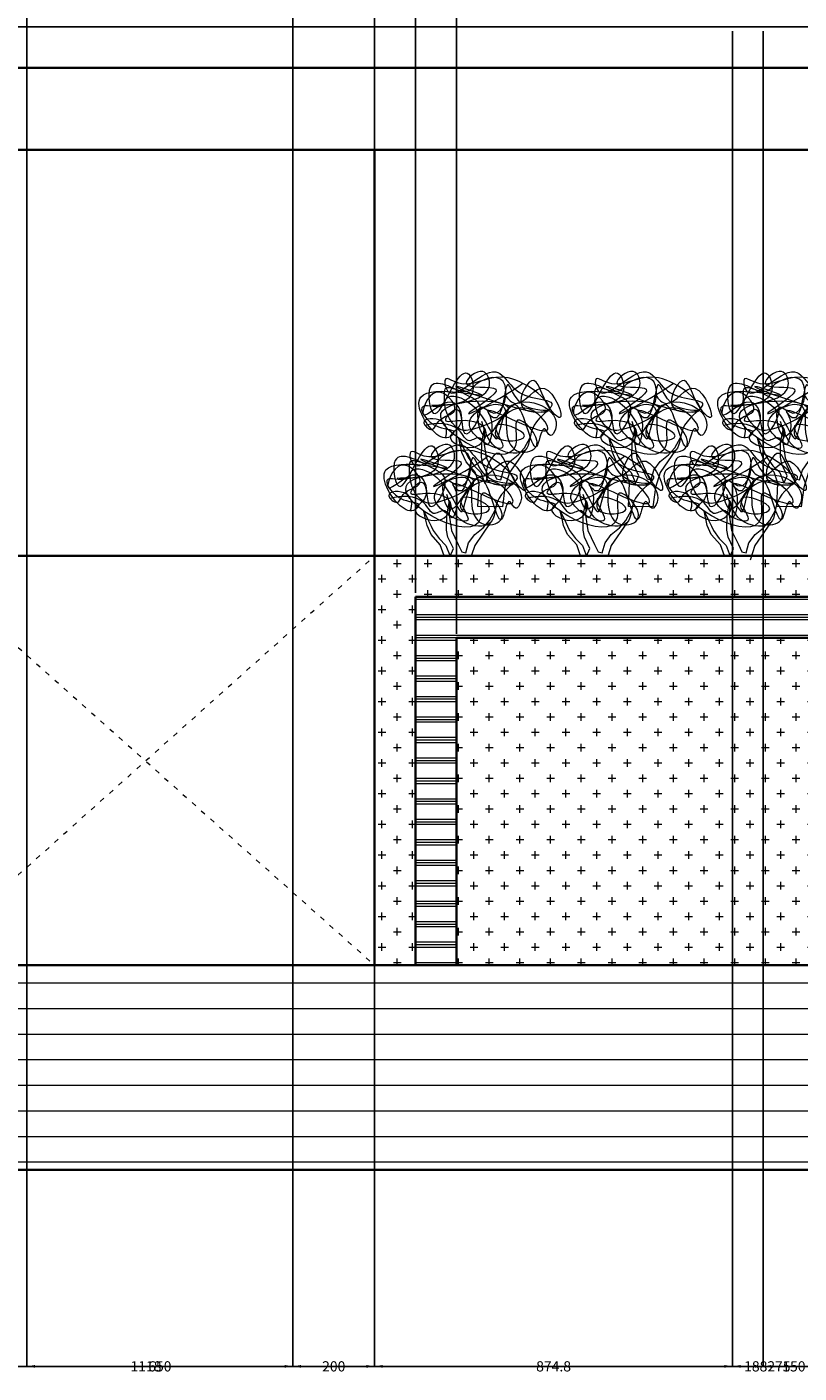
# Model space of a CAD drawing. Units: millimetres. Extents: x -692 to 9639, y -141 to 10345.
# Tile 6 of 19: x 6042 to 7929, y -141 to 3148. Entities that reach past the tile are written whole.
import ezdxf

# ---------------------------------------------------------------- set-up
doc = ezdxf.new("R2010")
doc.units = ezdxf.units.MM
doc.header["$MEASUREMENT"] = 0
doc.linetypes.add('ACAD_ISO03W100', pattern=[30, 12, -18])
for name, color, linetype, lineweight in [('A-ANNO-DIMS', 2, 'Continuous', 18), ('A-DOOR-SWNG', 3, 'ACAD_ISO03W100', 18), ('A-ELEV', 7, 'Continuous', 35), ('A-ELEV-PATT', 8, 'Continuous', 13), ('L-PLNT', 3, 'Continuous', 18)]:
    doc.layers.add(name, color=color, linetype=linetype, lineweight=lineweight)
doc.styles.get("Standard").update_dxf_attribs({"font": 'arial.ttf'})
doc.dimstyles.get("Standard").update_dxf_attribs({"dimtxt": 25, "dimasz": 20, "dimexe": 0.18, "dimexo": 10, "dimgap": 10, "dimtad": 0, "dimtih": 1, "dimtoh": 1, "dimdec": 0, "dimzin": 0, "dimdsep": 46, "dimtxsty": 'Standard', "dimcen": 10, "dimadec": 0, "dimazin": 0, "dimtfac": 1, "dimtdec": 0, "dimtofl": 0, "dimtmove": 0, "dimatfit": 3, "dimfxl": 1, "dimtolj": 1, "dimtzin": 0, "dimarcsym": 0})

# ---------------------------------------------------------------- blocks, each defined once
blk = doc.blocks.new('SHRUB-A')
for p, q in [((4.3, 148.6), (0, 167.6)), ((0, 167.6), (10, 146.8)), ((56.2, 156.7), (63.1, 192.4)), ((63.1, 192.4), (61.6, 157.6)), ((160.6, 144.2), (174.3, 169.5)), ((7.9, 132.5), (4.3, 148.6)), ((17.8, 109.9), (7.9, 132.5)), ((10, 146.8), (18, 130.3)), ((55.6, 120.9), (56.2, 156.7)), ((61.6, 157.6), (67.3, 119.6)), ((162.4, 138.4), (124.4, 83.7)), ((145.1, 126.5), (160.6, 144.2)), ((40.2, 84.8), (17.8, 109.9)), ((18, 130.3), (22.9, 120.3)), ((22.9, 120.3), (37.4, 100.1)), ((37.4, 100.1), (54, 83.6)), ((59.1, 104.1), (55.6, 120.9)), ((72.4, 75.8), (59.1, 104.1)), ((67.3, 119.6), (83.9, 86)), ((109.4, 89.7), (124.8, 110.5)), ((124.8, 110.5), (145.1, 126.5)), ((49.7, 57.7), (40.2, 84.8)), ((54, 83.6), (64.1, 57.4)), ((64.1, 57.4), (72.4, 75.8)), ((83.9, 86), (92.7, 68.2)), ((92.7, 68.2), (102.6, 65.4)), ((102.6, 65.4), (109.4, 89.7)), ((124.4, 83.7), (113, 47.4)), ((47, 0.4), (49.7, 57.7)), ((113, 47.4), (106.7, 0)), ((106.7, 0), (47, 0.4))]:
    blk.add_line(p, q)
blk = doc.blocks.new('SHRUB-B')
for p, q in [((56.2, 99.2), (63.1, 135)), ((63.1, 135), (61.6, 100.2)), ((4.3, 91.2), (0, 110.2)), ((0, 110.2), (10, 89.4)), ((55.6, 63.5), (56.2, 99.2)), ((61.6, 100.2), (67.3, 62.2)), ((160.6, 86.8), (174.3, 112.1)), ((7.9, 75.1), (4.3, 91.2)), ((17.8, 52.5), (7.9, 75.1)), ((10, 89.4), (18, 72.9)), ((18, 72.9), (22.9, 62.9)), ((124.8, 53.1), (145.1, 69.1)), ((145.1, 69.1), (160.6, 86.8)), ((40.2, 27.4), (17.8, 52.5)), ((22.9, 62.9), (37.4, 42.7)), ((37.4, 42.7), (54, 26.2)), ((59.1, 46.7), (55.6, 63.5)), ((72.4, 18.4), (59.1, 46.7)), ((67.3, 62.2), (83.9, 28.6)), ((109.4, 32.3), (124.8, 53.1)), ((49.7, 0.3), (40.2, 27.4)), ((54, 26.2), (64.1, 0)), ((64.1, 0), (72.4, 18.4)), ((83.9, 28.6), (92.7, 10.8)), ((92.7, 10.8), (102.6, 8)), ((102.6, 8), (109.4, 32.3))]:
    blk.add_line(p, q)
blk = doc.blocks.new('*D6')
at = {"layer": 'A-ANNO-DIMS', "color": 0, "lineweight": -2, "transparency": 16777216}
for p, q in [((2473.7, 345.6), (2473.7, -124.6)), ((9073.7, 345.6), (9073.7, -124.6)), ((2493.7, -124.4), (5726.4, -124.4)), ((9053.7, -124.4), (5821.1, -124.4))]:
    blk.add_line(p, q, dxfattribs=at)
at = {"layer": 'A-ANNO-DIMS', "color": 0, "lineweight": -3, "transparency": 16777216}
for points in [[(2493.7, -121.1), (2493.7, -127.8), (2473.7, -124.4)], [(9053.7, -121.1), (9053.7, -127.8), (9073.7, -124.4)]]:
    blk.add_solid(points, dxfattribs=at)
at = {"layer": 'Defpoints', "color": 0, "lineweight": -3, "transparency": 16777216}
for p in [(2473.7, 355.6), (9073.7, 355.6), (9073.7, -124.4)]:
    blk.add_point(p, dxfattribs=at)
at = {"layer": 'A-ANNO-DIMS', "color": 0, "transparency": 16777216, "insert": (5773.7, -124.4), "char_height": 25, "attachment_point": 5}
blk.add_mtext('\\A1;6600', dxfattribs=at)
blk = doc.blocks.new('*D7')
at = {"layer": 'A-ANNO-DIMS', "color": 0, "lineweight": -2, "transparency": 16777216}
for p, q in [((8481.5, 9848.8), (-649.1, 9848.8)), ((-648.9, 9828.8), (-648.9, 5124.9)), ((-648.9, 375.6), (-648.9, 5079.4)), ((2463.7, 355.6), (-649.1, 355.6))]:
    blk.add_line(p, q, dxfattribs=at)
at = {"layer": 'A-ANNO-DIMS', "color": 0, "lineweight": -3, "transparency": 16777216}
for points in [[(-652.2, 9828.8), (-645.6, 9828.8), (-648.9, 9848.8)], [(-652.2, 375.6), (-645.6, 375.6), (-648.9, 355.6)]]:
    blk.add_solid(points, dxfattribs=at)
at = {"layer": 'Defpoints', "color": 0, "lineweight": -3, "transparency": 16777216}
for p in [(-648.9, 9848.8), (8491.5, 9848.8), (2473.7, 355.6)]:
    blk.add_point(p, dxfattribs=at)
at = {"layer": 'A-ANNO-DIMS', "color": 0, "transparency": 16777216, "insert": (-648.9, 5102.2), "char_height": 25, "attachment_point": 5}
blk.add_mtext('\\A1;9493', dxfattribs=at)
blk = doc.blocks.new('*D22')
at = {"layer": 'A-ANNO-DIMS', "color": 0, "lineweight": -2, "transparency": 16777216}
for p, q in [((5773.7, 845.6), (5773.7, -124.6)), ((6891.7, 845.6), (6891.7, -124.6)), ((5793.7, -124.4), (6286.6, -124.4)), ((6871.7, -124.4), (6378.9, -124.4))]:
    blk.add_line(p, q, dxfattribs=at)
at = {"layer": 'A-ANNO-DIMS', "color": 0, "lineweight": -3, "transparency": 16777216}
for points in [[(5793.7, -121.1), (5793.7, -127.8), (5773.7, -124.4)], [(6871.7, -121.1), (6871.7, -127.8), (6891.7, -124.4)]]:
    blk.add_solid(points, dxfattribs=at)
at = {"layer": 'Defpoints', "color": 0, "lineweight": -3, "transparency": 16777216}
for p in [(5773.7, 855.6), (6891.7, 855.6), (6891.7, -124.4)]:
    blk.add_point(p, dxfattribs=at)
at = {"layer": 'A-ANNO-DIMS', "color": 0, "transparency": 16777216, "insert": (6332.7, -124.4), "char_height": 25, "attachment_point": 5}
blk.add_mtext('\\A1;1118', dxfattribs=at)
blk = doc.blocks.new('*D23')
at = {"layer": 'A-ANNO-DIMS', "color": 0, "lineweight": -2, "transparency": 16777216}
for p, q in [((6891.7, 845.6), (6891.7, -124.6)), ((8773.7, 845.6), (8773.7, -124.6)), ((6911.7, -124.4), (7786.7, -124.4)), ((8753.7, -124.4), (7878.8, -124.4))]:
    blk.add_line(p, q, dxfattribs=at)
at = {"layer": 'A-ANNO-DIMS', "color": 0, "lineweight": -3, "transparency": 16777216}
for points in [[(6911.7, -121.1), (6911.7, -127.8), (6891.7, -124.4)], [(8753.7, -121.1), (8753.7, -127.8), (8773.7, -124.4)]]:
    blk.add_solid(points, dxfattribs=at)
at = {"layer": 'Defpoints', "color": 0, "lineweight": -3, "transparency": 16777216}
for p in [(6891.7, 855.6), (8773.7, 855.6), (8773.7, -124.4)]:
    blk.add_point(p, dxfattribs=at)
at = {"layer": 'A-ANNO-DIMS', "color": 0, "transparency": 16777216, "insert": (7832.7, -124.4), "char_height": 25, "attachment_point": 5}
blk.add_mtext('\\A1;1882', dxfattribs=at)
blk = doc.blocks.new('*D32')
at = {"layer": 'A-ANNO-DIMS', "color": 0, "lineweight": -2, "transparency": 16777216}
for p, q in [((6871.7, 10328.8), (6851.7, 10328.8)), ((6891.7, 1865.6), (6891.7, 10329)), ((6991.7, 1765.6), (6991.7, 10329)), ((7011.7, 10328.8), (7031.7, 10328.8))]:
    blk.add_line(p, q, dxfattribs=at)
at = {"layer": 'A-ANNO-DIMS', "color": 0, "lineweight": -3, "transparency": 16777216}
for points in [[(6871.7, 10332.1), (6871.7, 10325.4), (6891.7, 10328.8)], [(7011.7, 10332.1), (7011.7, 10325.4), (6991.7, 10328.8)]]:
    blk.add_solid(points, dxfattribs=at)
at = {"layer": 'Defpoints', "color": 0, "lineweight": -3, "transparency": 16777216}
for p in [(6991.7, 10328.8), (6891.7, 1855.6), (6991.7, 1755.6)]:
    blk.add_point(p, dxfattribs=at)
at = {"layer": 'A-ANNO-DIMS', "color": 0, "transparency": 16777216, "insert": (6941.7, 10328.8), "char_height": 25, "attachment_point": 5}
blk.add_mtext('\\A1;100', dxfattribs=at)
blk = doc.blocks.new('*D33')
at = {"layer": 'A-ANNO-DIMS', "color": 0, "lineweight": -2, "transparency": 16777216}
for p, q in [((6971.7, 10328.8), (6951.7, 10328.8)), ((6991.7, 1765.6), (6991.7, 10329)), ((7091.7, 1665.6), (7091.7, 10329)), ((7111.7, 10328.8), (7131.7, 10328.8))]:
    blk.add_line(p, q, dxfattribs=at)
at = {"layer": 'A-ANNO-DIMS', "color": 0, "lineweight": -3, "transparency": 16777216}
for points in [[(6971.7, 10332.1), (6971.7, 10325.4), (6991.7, 10328.8)], [(7111.7, 10332.1), (7111.7, 10325.4), (7091.7, 10328.8)]]:
    blk.add_solid(points, dxfattribs=at)
at = {"layer": 'Defpoints', "color": 0, "lineweight": -3, "transparency": 16777216}
for p in [(7091.7, 10328.8), (6991.7, 1755.6), (7091.7, 1655.6)]:
    blk.add_point(p, dxfattribs=at)
at = {"layer": 'A-ANNO-DIMS', "color": 0, "transparency": 16777216, "insert": (7041.7, 10328.8), "char_height": 25, "attachment_point": 5}
blk.add_mtext('\\A1;100', dxfattribs=at)
blk = doc.blocks.new('*D34')
at = {"layer": 'A-ANNO-DIMS', "color": 0, "lineweight": -2, "transparency": 16777216}
for p, q in [((7091.7, 1665.6), (7091.7, 10329)), ((7111.7, 10328.8), (7786.7, 10328.8)), ((8553.7, 10328.8), (7878.8, 10328.8)), ((8573.7, 1665.6), (8573.7, 10329))]:
    blk.add_line(p, q, dxfattribs=at)
at = {"layer": 'A-ANNO-DIMS', "color": 0, "lineweight": -3, "transparency": 16777216}
for points in [[(7111.7, 10332.1), (7111.7, 10325.4), (7091.7, 10328.8)], [(8553.7, 10332.1), (8553.7, 10325.4), (8573.7, 10328.8)]]:
    blk.add_solid(points, dxfattribs=at)
at = {"layer": 'Defpoints', "color": 0, "lineweight": -3, "transparency": 16777216}
for p in [(8573.7, 10328.8), (7091.7, 1655.6), (8573.7, 1655.6)]:
    blk.add_point(p, dxfattribs=at)
at = {"layer": 'A-ANNO-DIMS', "color": 0, "transparency": 16777216, "insert": (7832.7, 10328.8), "char_height": 25, "attachment_point": 5}
blk.add_mtext('\\A1;1482', dxfattribs=at)
blk = doc.blocks.new('*D42')
at = {"layer": 'A-ANNO-DIMS', "color": 0, "lineweight": -2, "transparency": 16777216}
for p, q in [((6041.7, 3588.3), (6041.7, -124.6)), ((6691.7, 3588.3), (6691.7, -124.6)), ((6061.7, -124.4), (6329.1, -124.4)), ((6671.7, -124.4), (6404.4, -124.4))]:
    blk.add_line(p, q, dxfattribs=at)
at = {"layer": 'A-ANNO-DIMS', "color": 0, "lineweight": -3, "transparency": 16777216}
for points in [[(6061.7, -121.1), (6061.7, -127.8), (6041.7, -124.4)], [(6671.7, -121.1), (6671.7, -127.8), (6691.7, -124.4)]]:
    blk.add_solid(points, dxfattribs=at)
at = {"layer": 'Defpoints', "color": 0, "lineweight": -3, "transparency": 16777216}
for p in [(6041.7, 3598.3), (6691.7, 3598.3), (6691.7, -124.4)]:
    blk.add_point(p, dxfattribs=at)
at = {"layer": 'A-ANNO-DIMS', "color": 0, "transparency": 16777216, "insert": (6366.7, -124.4), "char_height": 25, "attachment_point": 5}
blk.add_mtext('\\A1;650', dxfattribs=at)
blk = doc.blocks.new('*D43')
at = {"layer": 'A-ANNO-DIMS', "color": 0, "lineweight": -2, "transparency": 16777216}
for p, q in [((6691.7, 3588.3), (6691.7, -124.6)), ((6891.7, 3588.3), (6891.7, -124.6)), ((6711.7, -124.4), (6754, -124.4)), ((6871.7, -124.4), (6829.5, -124.4))]:
    blk.add_line(p, q, dxfattribs=at)
at = {"layer": 'A-ANNO-DIMS', "color": 0, "lineweight": -3, "transparency": 16777216}
for points in [[(6711.7, -121.1), (6711.7, -127.8), (6691.7, -124.4)], [(6871.7, -121.1), (6871.7, -127.8), (6891.7, -124.4)]]:
    blk.add_solid(points, dxfattribs=at)
at = {"layer": 'Defpoints', "color": 0, "lineweight": -3, "transparency": 16777216}
for p in [(6691.7, 3598.3), (6891.7, 3598.3), (6891.7, -124.4)]:
    blk.add_point(p, dxfattribs=at)
at = {"layer": 'A-ANNO-DIMS', "color": 0, "transparency": 16777216, "insert": (6791.7, -124.4), "char_height": 25, "attachment_point": 5}
blk.add_mtext('\\A1;200', dxfattribs=at)
blk = doc.blocks.new('*D44')
at = {"layer": 'A-ANNO-DIMS', "color": 0, "lineweight": -2, "transparency": 16777216}
for p, q in [((6891.7, 3588.3), (6891.7, -124.6)), ((7766.5, 3138.3), (7766.5, -124.6)), ((6911.7, -124.4), (7276.9, -124.4)), ((7746.5, -124.4), (7381.4, -124.4))]:
    blk.add_line(p, q, dxfattribs=at)
at = {"layer": 'A-ANNO-DIMS', "color": 0, "lineweight": -3, "transparency": 16777216}
for points in [[(6911.7, -121.1), (6911.7, -127.8), (6891.7, -124.4)], [(7746.5, -121.1), (7746.5, -127.8), (7766.5, -124.4)]]:
    blk.add_solid(points, dxfattribs=at)
at = {"layer": 'Defpoints', "color": 0, "lineweight": -3, "transparency": 16777216}
for p in [(6891.7, 3598.3), (7766.5, 3148.3), (7766.5, -124.4)]:
    blk.add_point(p, dxfattribs=at)
at = {"layer": 'A-ANNO-DIMS', "color": 0, "transparency": 16777216, "insert": (7329.1, -124.4), "char_height": 25, "attachment_point": 5}
blk.add_mtext('\\A1;874.8', dxfattribs=at)
blk = doc.blocks.new('*D45')
at = {"layer": 'A-ANNO-DIMS', "color": 0, "lineweight": -2, "transparency": 16777216}
for p, q in [((7766.5, 3138.3), (7766.5, -124.6)), ((7841.5, 3138.3), (7841.5, -124.6)), ((7786.5, -124.4), (7821.5, -124.4)), ((7841.5, -124.4), (7861.5, -124.4))]:
    blk.add_line(p, q, dxfattribs=at)
at = {"layer": 'A-ANNO-DIMS', "color": 0, "lineweight": -3, "transparency": 16777216}
for points in [[(7786.5, -121.1), (7786.5, -127.8), (7766.5, -124.4)], [(7821.5, -121.1), (7821.5, -127.8), (7841.5, -124.4)]]:
    blk.add_solid(points, dxfattribs=at)
at = {"layer": 'Defpoints', "color": 0, "lineweight": -3, "transparency": 16777216}
for p in [(7766.5, 3148.3), (7841.5, 3148.3), (7841.5, -124.4)]:
    blk.add_point(p, dxfattribs=at)
at = {"layer": 'A-ANNO-DIMS', "color": 0, "transparency": 16777216, "insert": (7889.4, -124.4), "char_height": 25, "attachment_point": 5}
blk.add_mtext('\\A1;75', dxfattribs=at)
blk = doc.blocks.new('*D46')
at = {"layer": 'A-ANNO-DIMS', "color": 0, "lineweight": -2, "transparency": 16777216}
for p, q in [((7841.5, 3138.3), (7841.5, -124.6)), ((7991.5, 3138.3), (7991.5, -124.6)), ((7861.5, -124.4), (7880.1, -124.4)), ((7971.5, -124.4), (7952.9, -124.4))]:
    blk.add_line(p, q, dxfattribs=at)
at = {"layer": 'A-ANNO-DIMS', "color": 0, "lineweight": -3, "transparency": 16777216}
for points in [[(7861.5, -121.1), (7861.5, -127.8), (7841.5, -124.4)], [(7971.5, -121.1), (7971.5, -127.8), (7991.5, -124.4)]]:
    blk.add_solid(points, dxfattribs=at)
at = {"layer": 'Defpoints', "color": 0, "lineweight": -3, "transparency": 16777216}
for p in [(7841.5, 3148.3), (7991.5, 3148.3), (7991.5, -124.4)]:
    blk.add_point(p, dxfattribs=at)
at = {"layer": 'A-ANNO-DIMS', "color": 0, "transparency": 16777216, "insert": (7916.5, -124.4), "char_height": 25, "attachment_point": 5}
blk.add_mtext('\\A1;150', dxfattribs=at)
blk = doc.blocks.new('*D71')
at = {"layer": 'A-ANNO-DIMS', "color": 0, "lineweight": -2, "transparency": 16777216}
for p, q in [((5201.5, 3598.3), (9553.9, 3598.3)), ((9553.7, 3578.3), (9553.7, 3396)), ((9553.7, 3168.3), (9553.7, 3350.5)), ((5101.5, 3148.3), (9553.9, 3148.3))]:
    blk.add_line(p, q, dxfattribs=at)
at = {"layer": 'A-ANNO-DIMS', "color": 0, "lineweight": -3, "transparency": 16777216}
for points in [[(9550.4, 3578.3), (9557.1, 3578.3), (9553.7, 3598.3)], [(9550.4, 3168.3), (9557.1, 3168.3), (9553.7, 3148.3)]]:
    blk.add_solid(points, dxfattribs=at)
at = {"layer": 'Defpoints', "color": 0, "lineweight": -3, "transparency": 16777216}
for p in [(5191.5, 3598.3), (9553.7, 3598.3), (5091.5, 3148.3)]:
    blk.add_point(p, dxfattribs=at)
at = {"layer": 'A-ANNO-DIMS', "color": 0, "transparency": 16777216, "insert": (9553.7, 3373.3), "char_height": 25, "attachment_point": 5}
blk.add_mtext('\\A1;450', dxfattribs=at)

msp = doc.modelspace()

# ---------------------------------------------------------------- hatches: boundary and pattern name
at = {"layer": 'A-ELEV-PATT'}
h = msp.add_hatch(dxfattribs=at)
h.set_pattern_fill('CROSS', color=256, scale=150)
h.paths.add_polyline_path([(8573.746, 1655.575), (7091.746, 1655.575), (7091.746, 855.575), (7273.746, 855.575), (8573.746, 855.575)], flags=17)
h.paths.add_polyline_path([(8773.746, 1855.575), (8463.966, 1855.575), (8463.828, 1855.268), (8463.709, 1855.575), (7761.103, 1855.575), (7760.965, 1855.268), (7760.846, 1855.575), (7409.705, 1855.575), (7409.567, 1855.268), (7409.448, 1855.575), (7076.174, 1855.575), (7076.035, 1855.268), (7075.916, 1855.575), (6891.746, 1855.575), (6891.746, 855.575), (6991.746, 855.575), (6991.746, 1755.575), (8673.746, 1755.575), (8673.746, 855.575), (8773.746, 855.575)])
h = msp.add_hatch(dxfattribs=at)
h.set_pattern_fill('PLAST', color=256, scale=200)
h.paths.add_polyline_path([(8673.746, 1755.575), (6991.746, 1755.575), (6991.746, 855.575), (7091.746, 855.575), (7091.746, 1655.575), (8573.746, 1655.575), (8573.746, 855.575), (8673.746, 855.575)])
h = msp.add_hatch(dxfattribs=at)
h.set_pattern_fill('LINE', color=256, scale=500)
h.paths.add_polyline_path([(9073.746, 855.575), (8773.746, 855.575), (7273.746, 855.575), (2773.746, 855.575), (2473.746, 855.575), (2473.746, 355.575), (9073.746, 355.575)])

# ---------------------------------------------------------------- linework, layer by layer
at = {"layer": 'A-DOOR-SWNG'}
for p, q in [((5773.746, 855.575), (6891.746, 1855.575)), ((5773.746, 1851.922), (6891.746, 855.575))]:
    msp.add_line(p, q, dxfattribs=at)
at = {"layer": 'A-ELEV'}
for p, q in [((5191.547, 3048.27), (8491.547, 3048.27)), ((5773.746, 2848.27), (8341.547, 2848.27)), ((6891.746, 1855.575), (6891.746, 2848.27)), ((6891.746, 1855.575), (5773.746, 1855.575)), ((8773.746, 1855.575), (6891.746, 1855.575)), ((6891.746, 1855.575), (6891.746, 855.575)), ((6991.746, 1755.575), (6991.746, 855.575)), ((8673.746, 1755.575), (6991.746, 1755.575)), ((7091.746, 1655.575), (7091.746, 855.575)), ((8573.746, 1655.575), (7091.746, 1655.575)), ((7273.746, 855.575), (2773.746, 855.575)), ((7273.746, 855.575), (8773.746, 855.575)), ((2473.746, 355.575), (9073.746, 355.575))]:
    msp.add_line(p, q, dxfattribs=at)
at = {"layer": 'L-PLNT'}
for p, q in [((7174.339, 1936.243), (7136.274, 1881.512)), ((7507.871, 1936.243), (7469.806, 1881.512)), ((7859.269, 1936.243), (7821.204, 1881.512)), ((7136.274, 1881.512), (7128.698, 1857.344)), ((7469.806, 1881.512), (7462.229, 1857.344)), ((7821.204, 1881.512), (7809.854, 1845.31))]:
    msp.add_line(p, q, dxfattribs=at)
for points, knots in [([(7210.912, 2249.042), (7217.418, 2237.706), (7250.654, 2207.754), (7307.084, 2319.362), (7366.264, 2167.67), (7301.628, 2229.166), (7285.902, 2328.371), (7218.943, 2194.758), (7356.409, 2215.079), (7239.565, 2204.712), (7210.229, 2329.754), (7204.627, 2163.076), (7152.125, 2224.979), (7245.806, 2179.391), (7342.871, 2141.303), (7273.71, 2230.619), (7207.557, 2210.89), (7165.346, 2127.262), (7316.233, 2141.658), (7150.625, 2203.471), (7246.999, 2083.661), (7053.157, 2177.336), (7227.853, 2256.385), (7205.644, 2158.211), (7234.382, 2098.948), (7320.634, 2123.83), (7218.8, 2228.342), (7274.006, 2029.162), (6888.412, 2240.289), (7303.506, 2243.554), (7153.523, 2166.62), (7082.671, 2156.226), (7039.859, 2264.065), (7154.64, 2230.339), (7196.727, 2085.9), (7201.713, 2275.464), (7363.406, 2209.432), (7320.679, 2140.066), (7302.642, 2187.643), (7281.847, 2051.748), (7245.094, 2333.663), (7157.962, 2070.375), (7132.961, 2246.68), (7202.729, 2175.732), (7234.396, 2316.142), (7143.856, 2285.782), (7114.73, 2244.752), (7047.788, 2291.151), (7073.979, 2204.577), (6981.537, 2240.713), (7031.353, 2161.604), (7092.873, 2165.76), (7062.706, 2127.131), (7007.402, 2181.977), (6983.121, 2288.868), (7227.495, 2226.655), (6979.203, 2307.83), (7439.953, 2128.857), (7214.288, 2328.1), (7134.444, 2267.378), (7088.142, 2280.064), (7060.058, 2295.919), (7072.42, 2206.055), (7173.748, 2346.33), (7225.888, 2266.58), (7264.702, 2241.096), (7356.378, 2233.207), (7263.361, 2180.878), (7277.522, 2100.111), (7177.704, 2108.211), (7162.078, 2156.893), (7153.334, 2184.132)], [2413.81083439, 2413.81083439, 2413.81083439, 2413.81083439, 2446.13175162, 2525.76080664, 2606.35842411, 2641.00152553, 2720.74212251, 2790.99014926, 2851.81652626, 2913.32865241, 2976.26621652, 3063.90114016, 3082.75198237, 3142.42040078, 3234.21047015, 3290.89514405, 3366.44484787, 3415.98940505, 3483.69911772, 3557.93307926, 3609.73318023, 3705.73947781, 3799.4035149, 3865.9559372, 3923.0506034, 3967.47996902, 4044.49288828, 4106.44083814, 4304.51898163, 4470.20683119, 4567.66187689, 4605.3795614, 4686.71522755, 4750.59418277, 4853.67923318, 4940.38216709, 5061.92671957, 5081.75583403, 5102.38342504, 5145.20608443, 5257.20859169, 5364.77120979, 5434.601162, 5468.93345211, 5548.91442162, 5624.29444335, 5636.24531967, 5696.20028889, 5735.53268567, 5783.76480276, 5846.42206129, 5886.03768999, 5892.5373904, 5975.51315878, 6025.10951571, 6171.93373357, 6229.50952465, 6457.88730992, 6585.61219414, 6694.59236697, 6720.94216912, 6740.48817363, 6762.80712224, 6890.45590486, 6938.76737224, 6996.52597549, 7050.2147859, 7119.04318667, 7183.57042671, 7247.02609863, 7327.63038966, 7327.63038966, 7327.63038966, 7327.63038966]), ([(7064.221, 2143.94), (7070.284, 2158.144), (7066.79, 2196.249), (6992.219, 2191.386), (7035.666, 2154.108), (7046.348, 2198.183), (7115.409, 2201.259), (7035.457, 2293.571), (6986.961, 2156.7), (7085.437, 2271.959), (7117.212, 2174.361), (7053.159, 2143.553), (7135.962, 2102.288), (7183.308, 2169.843), (7118.862, 2193.667), (7048.32, 2176.214), (7109.825, 2245.325), (7096.88, 2104.492), (7171.192, 2221.171), (7105.428, 2254.125), (7009.652, 2308.243), (7033.817, 2163.685), (7073.391, 2260.33), (7120.527, 2324.908), (7154.118, 2215.034), (6925.37, 2230.018), (7199.519, 2217.011), (7159.517, 2326.244), (7076.118, 2255.543), (7251.153, 2284.242), (7039.629, 2159.222), (7203.882, 2239.906), (7254.013, 2277.481)], [369.05069933, 369.05069933, 369.05069933, 369.05069933, 408.0755152, 451.81999766, 477.70991819, 501.76804774, 551.72688153, 614.71506468, 677.59190345, 752.65992621, 814.92518896, 848.06947292, 911.78367098, 957.89252981, 1028.01014559, 1063.15062915, 1099.93333455, 1162.00574744, 1235.23981988, 1278.45742209, 1371.86548038, 1434.47491944, 1513.90135623, 1562.79289697, 1613.81915843, 1716.27616866, 1864.9556669, 1902.31221643, 1951.61463942, 2025.20033993, 2111.30740148, 2244.75178922, 2244.75178922, 2244.75178922, 2244.75178922]), ([(7578.761, 2249.042), (7585.267, 2237.706), (7618.503, 2207.754), (7674.932, 2319.362), (7734.113, 2167.67), (7669.477, 2229.166), (7653.751, 2328.371), (7586.792, 2194.758), (7724.258, 2215.079), (7607.413, 2204.712), (7578.078, 2329.754), (7572.475, 2163.076), (7519.974, 2224.979), (7613.654, 2179.391), (7710.72, 2141.303), (7641.559, 2230.619), (7575.406, 2210.89), (7533.195, 2127.262), (7684.082, 2141.658), (7518.473, 2203.471), (7614.847, 2083.661), (7421.005, 2177.336), (7595.702, 2256.385), (7573.493, 2158.211), (7602.23, 2098.948), (7688.483, 2123.83), (7586.649, 2228.342), (7641.854, 2029.162), (7256.261, 2240.289), (7671.354, 2243.554), (7521.371, 2166.62), (7450.52, 2156.226), (7407.707, 2264.065), (7522.488, 2230.339), (7564.576, 2085.9), (7569.562, 2275.464), (7731.255, 2209.432), (7688.528, 2140.066), (7670.491, 2187.643), (7649.696, 2051.748), (7612.942, 2333.663), (7525.811, 2070.375), (7500.809, 2246.68), (7570.578, 2175.732), (7602.245, 2316.142), (7511.705, 2285.782), (7482.579, 2244.752), (7415.637, 2291.151), (7441.828, 2204.577), (7349.386, 2240.713), (7399.202, 2161.604), (7460.722, 2165.76), (7430.555, 2127.131), (7375.251, 2181.977), (7350.97, 2288.868), (7595.344, 2226.655), (7347.052, 2307.83), (7807.801, 2128.857), (7582.137, 2328.1), (7502.293, 2267.378), (7455.991, 2280.064), (7427.907, 2295.919), (7440.268, 2206.055), (7541.597, 2346.33), (7593.737, 2266.58), (7632.551, 2241.096), (7724.227, 2233.207), (7631.21, 2180.878), (7645.371, 2100.111), (7545.553, 2108.211), (7529.927, 2156.893), (7521.183, 2184.132)], [2413.81083439, 2413.81083439, 2413.81083439, 2413.81083439, 2446.13175162, 2525.76080664, 2606.35842411, 2641.00152553, 2720.74212251, 2790.99014926, 2851.81652626, 2913.32865241, 2976.26621652, 3063.90114016, 3082.75198237, 3142.42040078, 3234.21047015, 3290.89514405, 3366.44484787, 3415.98940505, 3483.69911772, 3557.93307926, 3609.73318023, 3705.73947781, 3799.4035149, 3865.9559372, 3923.0506034, 3967.47996902, 4044.49288828, 4106.44083814, 4304.51898163, 4470.20683119, 4567.66187689, 4605.3795614, 4686.71522755, 4750.59418277, 4853.67923318, 4940.38216709, 5061.92671957, 5081.75583403, 5102.38342504, 5145.20608443, 5257.20859169, 5364.77120979, 5434.601162, 5468.93345211, 5548.91442162, 5624.29444335, 5636.24531967, 5696.20028889, 5735.53268567, 5783.76480276, 5846.42206129, 5886.03768999, 5892.5373904, 5975.51315878, 6025.10951571, 6171.93373357, 6229.50952465, 6457.88730992, 6585.61219414, 6694.59236697, 6720.94216912, 6740.48817363, 6762.80712224, 6890.45590486, 6938.76737224, 6996.52597549, 7050.2147859, 7119.04318667, 7183.57042671, 7247.02609863, 7327.63038966, 7327.63038966, 7327.63038966, 7327.63038966]), ([(7432.07, 2143.94), (7438.133, 2158.144), (7434.639, 2196.249), (7360.067, 2191.386), (7403.515, 2154.108), (7414.197, 2198.183), (7483.258, 2201.259), (7403.306, 2293.571), (7354.81, 2156.7), (7453.286, 2271.959), (7485.061, 2174.361), (7421.007, 2143.553), (7503.81, 2102.288), (7551.157, 2169.843), (7486.711, 2193.667), (7416.169, 2176.214), (7477.674, 2245.325), (7464.729, 2104.492), (7539.04, 2221.171), (7473.277, 2254.125), (7377.501, 2308.243), (7401.666, 2163.685), (7441.24, 2260.33), (7488.376, 2324.908), (7521.967, 2215.034), (7293.219, 2230.018), (7567.367, 2217.011), (7527.366, 2326.244), (7443.967, 2255.543), (7619.002, 2284.242), (7407.478, 2159.222), (7571.731, 2239.906), (7621.862, 2277.481)], [369.05069933, 369.05069933, 369.05069933, 369.05069933, 408.0755152, 451.81999766, 477.70991819, 501.76804774, 551.72688153, 614.71506468, 677.59190345, 752.65992621, 814.92518896, 848.06947292, 911.78367098, 957.89252981, 1028.01014559, 1063.15062915, 1099.93333455, 1162.00574744, 1235.23981988, 1278.45742209, 1371.86548038, 1434.47491944, 1513.90135623, 1562.79289697, 1613.81915843, 1716.27616866, 1864.9556669, 1902.31221643, 1951.61463942, 2025.20033993, 2111.30740148, 2244.75178922, 2244.75178922, 2244.75178922, 2244.75178922]), ([(7941.428, 2249.042), (7947.933, 2237.706), (7981.169, 2207.754), (8037.599, 2319.362), (8096.779, 2167.67), (8032.143, 2229.166), (8016.418, 2328.371), (7949.459, 2194.758), (8086.925, 2215.079), (7970.08, 2204.712), (7940.744, 2329.754), (7935.142, 2163.076), (7882.64, 2224.979), (7976.321, 2179.391), (8073.386, 2141.303), (8004.226, 2230.619), (7938.072, 2210.89), (7895.861, 2127.262), (8046.749, 2141.658), (7881.14, 2203.471), (7977.514, 2083.661), (7783.672, 2177.336), (7958.368, 2256.385), (7936.159, 2158.211), (7964.897, 2098.948), (8051.149, 2123.83), (7949.315, 2228.342), (8004.521, 2029.162), (7618.927, 2240.289), (8034.021, 2243.554), (7884.038, 2166.62), (7813.186, 2156.226), (7770.374, 2264.065), (7885.155, 2230.339), (7927.243, 2085.9), (7932.228, 2275.464), (8093.922, 2209.432), (8051.195, 2140.066), (8033.158, 2187.643), (8012.363, 2051.748), (7975.609, 2333.663), (7888.478, 2070.375), (7863.476, 2246.68), (7933.245, 2175.732), (7964.912, 2316.142), (7874.371, 2285.782), (7845.246, 2244.752), (7778.303, 2291.151), (7804.494, 2204.577), (7712.052, 2240.713), (7761.869, 2161.604), (7823.388, 2165.76), (7793.222, 2127.131), (7737.918, 2181.977), (7713.636, 2288.868), (7958.01, 2226.655), (7709.719, 2307.83), (8170.468, 2128.857), (7944.803, 2328.1), (7864.96, 2267.378), (7818.657, 2280.064), (7790.573, 2295.919), (7802.935, 2206.055), (7904.263, 2346.33), (7956.403, 2266.58), (7995.218, 2241.096), (8086.893, 2233.207), (7993.877, 2180.878), (8008.037, 2100.111), (7908.22, 2108.211), (7892.593, 2156.893), (7883.85, 2184.132)], [2413.81083439, 2413.81083439, 2413.81083439, 2413.81083439, 2446.13175162, 2525.76080664, 2606.35842411, 2641.00152553, 2720.74212251, 2790.99014926, 2851.81652626, 2913.32865241, 2976.26621652, 3063.90114016, 3082.75198237, 3142.42040078, 3234.21047015, 3290.89514405, 3366.44484787, 3415.98940505, 3483.69911772, 3557.93307926, 3609.73318023, 3705.73947781, 3799.4035149, 3865.9559372, 3923.0506034, 3967.47996902, 4044.49288828, 4106.44083814, 4304.51898163, 4470.20683119, 4567.66187689, 4605.3795614, 4686.71522755, 4750.59418277, 4853.67923318, 4940.38216709, 5061.92671957, 5081.75583403, 5102.38342504, 5145.20608443, 5257.20859169, 5364.77120979, 5434.601162, 5468.93345211, 5548.91442162, 5624.29444335, 5636.24531967, 5696.20028889, 5735.53268567, 5783.76480276, 5846.42206129, 5886.03768999, 5892.5373904, 5975.51315878, 6025.10951571, 6171.93373357, 6229.50952465, 6457.88730992, 6585.61219414, 6694.59236697, 6720.94216912, 6740.48817363, 6762.80712224, 6890.45590486, 6938.76737224, 6996.52597549, 7050.2147859, 7119.04318667, 7183.57042671, 7247.02609863, 7327.63038966, 7327.63038966, 7327.63038966, 7327.63038966]), ([(7794.737, 2143.94), (7800.8, 2158.144), (7797.305, 2196.249), (7722.734, 2191.386), (7766.182, 2154.108), (7776.863, 2198.183), (7845.924, 2201.259), (7765.972, 2293.571), (7717.477, 2156.7), (7815.952, 2271.959), (7847.727, 2174.361), (7783.674, 2143.553), (7866.477, 2102.288), (7913.823, 2169.843), (7849.377, 2193.667), (7778.836, 2176.214), (7840.34, 2245.325), (7827.395, 2104.492), (7901.707, 2221.171), (7835.943, 2254.125), (7740.167, 2308.243), (7764.333, 2163.685), (7803.906, 2260.33), (7851.043, 2324.908), (7884.633, 2215.034), (7655.885, 2230.018), (7930.034, 2217.011), (7890.032, 2326.244), (7806.634, 2255.543), (7981.668, 2284.242), (7770.144, 2159.222), (7934.397, 2239.906), (7984.529, 2277.481)], [369.05069933, 369.05069933, 369.05069933, 369.05069933, 408.0755152, 451.81999766, 477.70991819, 501.76804774, 551.72688153, 614.71506468, 677.59190345, 752.65992621, 814.92518896, 848.06947292, 911.78367098, 957.89252981, 1028.01014559, 1063.15062915, 1099.93333455, 1162.00574744, 1235.23981988, 1278.45742209, 1371.86548038, 1434.47491944, 1513.90135623, 1562.79289697, 1613.81915843, 1716.27616866, 1864.9556669, 1902.31221643, 1951.61463942, 2025.20033993, 2111.30740148, 2244.75178922, 2244.75178922, 2244.75178922, 2244.75178922]), ([(7168.942, 2206.874), (7172.432, 2200.207), (7183.929, 2178.247), (7170.858, 2104.319), (7149.677, 2153.752), (7116.867, 2125.304), (7099.28, 2181.552), (7041.527, 2182.208), (7014.815, 2174.344)], [0, 0, 0, 0, 24.87287104, 81.92705424, 103.09014331, 128.64171207, 165.87657864, 231.33124244, 231.33124244, 231.33124244, 231.33124244]), ([(7536.791, 2206.874), (7540.281, 2200.207), (7551.778, 2178.247), (7538.707, 2104.319), (7517.526, 2153.752), (7484.715, 2125.304), (7467.129, 2181.552), (7409.376, 2182.208), (7382.664, 2174.344)], [0, 0, 0, 0, 24.87287104, 81.92705424, 103.09014331, 128.64171207, 165.87657864, 231.33124244, 231.33124244, 231.33124244, 231.33124244]), ([(7899.457, 2206.874), (7902.947, 2200.207), (7914.444, 2178.247), (7901.373, 2104.319), (7880.192, 2153.752), (7847.382, 2125.304), (7829.795, 2181.552), (7772.042, 2182.208), (7745.331, 2174.344)], [0, 0, 0, 0, 24.87287104, 81.92705424, 103.09014331, 128.64171207, 165.87657864, 231.33124244, 231.33124244, 231.33124244, 231.33124244]), ([(7125.562, 2070.999), (7132.068, 2059.664), (7165.304, 2029.712), (7221.733, 2141.319), (7280.914, 1989.627), (7216.277, 2051.123), (7200.552, 2150.328), (7133.593, 2016.716), (7271.059, 2037.036), (7154.214, 2026.669), (7124.879, 2151.711), (7119.276, 1985.034), (7066.774, 2046.936), (7160.455, 2001.348), (7257.521, 1963.26), (7188.36, 2052.576), (7122.207, 2032.847), (7079.995, 1949.219), (7230.883, 1963.615), (7065.274, 2025.428), (7161.648, 1905.618), (6967.806, 1999.293), (7142.503, 2078.342), (7120.294, 1980.168), (7149.031, 1920.905), (7235.284, 1945.788), (7133.449, 2050.299), (7188.655, 1851.119), (6803.062, 2062.246), (7218.155, 2065.511), (7068.172, 1988.577), (6997.32, 1978.184), (6954.508, 2086.023), (7069.289, 2052.296), (7111.377, 1907.857), (7116.362, 2097.422), (7278.056, 2031.389), (7235.329, 1962.023), (7217.292, 2009.601), (7196.497, 1873.705), (7159.743, 2155.62), (7072.612, 1892.333), (7047.61, 2068.637), (7117.379, 1997.689), (7149.046, 2138.099), (7058.506, 2107.74), (7029.38, 2066.709), (6962.438, 2113.109), (6988.628, 2026.534), (6896.187, 2062.67), (6946.003, 1983.561), (7007.523, 1987.717), (6977.356, 1949.089), (6922.052, 2003.934), (6897.77, 2110.825), (7142.145, 2048.612), (6893.853, 2129.787), (7354.602, 1950.814), (7128.937, 2150.057), (7049.094, 2089.335), (7002.791, 2102.021), (6974.707, 2117.876), (6987.069, 2028.012), (7088.398, 2168.287), (7140.538, 2088.537), (7179.352, 2063.053), (7271.028, 2055.164), (7178.011, 2002.836), (7192.172, 1922.068), (7092.354, 1930.168), (7076.728, 1978.85), (7067.984, 2006.089)], [2413.81083439, 2413.81083439, 2413.81083439, 2413.81083439, 2446.13175162, 2525.76080664, 2606.35842411, 2641.00152553, 2720.74212251, 2790.99014926, 2851.81652626, 2913.32865241, 2976.26621652, 3063.90114016, 3082.75198237, 3142.42040078, 3234.21047015, 3290.89514405, 3366.44484787, 3415.98940505, 3483.69911772, 3557.93307926, 3609.73318023, 3705.73947781, 3799.4035149, 3865.9559372, 3923.0506034, 3967.47996902, 4044.49288828, 4106.44083814, 4304.51898163, 4470.20683119, 4567.66187689, 4605.3795614, 4686.71522755, 4750.59418277, 4853.67923318, 4940.38216709, 5061.92671957, 5081.75583403, 5102.38342504, 5145.20608443, 5257.20859169, 5364.77120979, 5434.601162, 5468.93345211, 5548.91442162, 5624.29444335, 5636.24531967, 5696.20028889, 5735.53268567, 5783.76480276, 5846.42206129, 5886.03768999, 5892.5373904, 5975.51315878, 6025.10951571, 6171.93373357, 6229.50952465, 6457.88730992, 6585.61219414, 6694.59236697, 6720.94216912, 6740.48817363, 6762.80712224, 6890.45590486, 6938.76737224, 6996.52597549, 7050.2147859, 7119.04318667, 7183.57042671, 7247.02609863, 7327.63038966, 7327.63038966, 7327.63038966, 7327.63038966]), ([(6978.871, 1965.897), (6984.934, 1980.101), (6981.439, 2018.206), (6906.868, 2013.343), (6950.316, 1976.065), (6960.998, 2020.14), (7030.059, 2023.217), (6950.107, 2115.528), (6901.611, 1978.657), (7000.087, 2093.916), (7031.862, 1996.319), (6967.808, 1965.51), (7050.611, 1924.245), (7097.958, 1991.8), (7033.511, 2015.624), (6962.97, 1998.171), (7024.474, 2067.282), (7011.53, 1926.449), (7085.841, 2043.128), (7020.078, 2076.082), (6924.302, 2130.201), (6948.467, 1985.642), (6988.041, 2082.287), (7035.177, 2146.866), (7068.768, 2036.992), (6840.02, 2051.975), (7114.168, 2038.969), (7074.167, 2148.201), (6990.768, 2077.5), (7165.803, 2106.199), (6954.279, 1981.179), (7118.532, 2061.864), (7168.663, 2099.439)], [369.05069933, 369.05069933, 369.05069933, 369.05069933, 408.0755152, 451.81999766, 477.70991819, 501.76804774, 551.72688153, 614.71506468, 677.59190345, 752.65992621, 814.92518896, 848.06947292, 911.78367098, 957.89252981, 1028.01014559, 1063.15062915, 1099.93333455, 1162.00574744, 1235.23981988, 1278.45742209, 1371.86548038, 1434.47491944, 1513.90135623, 1562.79289697, 1613.81915843, 1716.27616866, 1864.9556669, 1902.31221643, 1951.61463942, 2025.20033993, 2111.30740148, 2244.75178922, 2244.75178922, 2244.75178922, 2244.75178922]), ([(7459.094, 2070.999), (7465.599, 2059.664), (7498.835, 2029.712), (7555.265, 2141.319), (7614.446, 1989.627), (7549.809, 2051.123), (7534.084, 2150.328), (7467.125, 2016.716), (7604.591, 2037.036), (7487.746, 2026.669), (7458.41, 2151.711), (7452.808, 1985.034), (7400.306, 2046.936), (7493.987, 2001.348), (7591.053, 1963.26), (7521.892, 2052.576), (7455.738, 2032.847), (7413.527, 1949.219), (7564.415, 1963.615), (7398.806, 2025.428), (7495.18, 1905.618), (7301.338, 1999.293), (7476.034, 2078.342), (7453.826, 1980.168), (7482.563, 1920.905), (7568.815, 1945.788), (7466.981, 2050.299), (7522.187, 1851.119), (7136.594, 2062.246), (7551.687, 2065.511), (7401.704, 1988.577), (7330.852, 1978.184), (7288.04, 2086.023), (7402.821, 2052.296), (7444.909, 1907.857), (7449.894, 2097.422), (7611.588, 2031.389), (7568.861, 1962.023), (7550.824, 2009.601), (7530.029, 1873.705), (7493.275, 2155.62), (7406.144, 1892.333), (7381.142, 2068.637), (7450.911, 1997.689), (7482.578, 2138.099), (7392.037, 2107.74), (7362.912, 2066.709), (7295.969, 2113.109), (7322.16, 2026.534), (7229.718, 2062.67), (7279.535, 1983.561), (7341.055, 1987.717), (7310.888, 1949.089), (7255.584, 2003.934), (7231.302, 2110.825), (7475.677, 2048.612), (7227.385, 2129.787), (7688.134, 1950.814), (7462.469, 2150.057), (7382.626, 2089.335), (7336.323, 2102.021), (7308.239, 2117.876), (7320.601, 2028.012), (7421.93, 2168.287), (7474.069, 2088.537), (7512.884, 2063.053), (7604.56, 2055.164), (7511.543, 2002.836), (7525.704, 1922.068), (7425.886, 1930.168), (7410.259, 1978.85), (7401.516, 2006.089)], [2413.81083439, 2413.81083439, 2413.81083439, 2413.81083439, 2446.13175162, 2525.76080664, 2606.35842411, 2641.00152553, 2720.74212251, 2790.99014926, 2851.81652626, 2913.32865241, 2976.26621652, 3063.90114016, 3082.75198237, 3142.42040078, 3234.21047015, 3290.89514405, 3366.44484787, 3415.98940505, 3483.69911772, 3557.93307926, 3609.73318023, 3705.73947781, 3799.4035149, 3865.9559372, 3923.0506034, 3967.47996902, 4044.49288828, 4106.44083814, 4304.51898163, 4470.20683119, 4567.66187689, 4605.3795614, 4686.71522755, 4750.59418277, 4853.67923318, 4940.38216709, 5061.92671957, 5081.75583403, 5102.38342504, 5145.20608443, 5257.20859169, 5364.77120979, 5434.601162, 5468.93345211, 5548.91442162, 5624.29444335, 5636.24531967, 5696.20028889, 5735.53268567, 5783.76480276, 5846.42206129, 5886.03768999, 5892.5373904, 5975.51315878, 6025.10951571, 6171.93373357, 6229.50952465, 6457.88730992, 6585.61219414, 6694.59236697, 6720.94216912, 6740.48817363, 6762.80712224, 6890.45590486, 6938.76737224, 6996.52597549, 7050.2147859, 7119.04318667, 7183.57042671, 7247.02609863, 7327.63038966, 7327.63038966, 7327.63038966, 7327.63038966]), ([(7312.403, 1965.897), (7318.466, 1980.101), (7314.971, 2018.206), (7240.4, 2013.343), (7283.848, 1976.065), (7294.529, 2020.14), (7363.59, 2023.217), (7283.638, 2115.528), (7235.143, 1978.657), (7333.618, 2093.916), (7365.394, 1996.319), (7301.34, 1965.51), (7384.143, 1924.245), (7431.49, 1991.8), (7367.043, 2015.624), (7296.502, 1998.171), (7358.006, 2067.282), (7345.062, 1926.449), (7419.373, 2043.128), (7353.609, 2076.082), (7257.834, 2130.201), (7281.999, 1985.642), (7321.572, 2082.287), (7368.709, 2146.866), (7402.3, 2036.992), (7173.552, 2051.975), (7447.7, 2038.969), (7407.699, 2148.201), (7324.3, 2077.5), (7499.334, 2106.199), (7287.81, 1981.179), (7452.063, 2061.864), (7502.195, 2099.439)], [369.05069933, 369.05069933, 369.05069933, 369.05069933, 408.0755152, 451.81999766, 477.70991819, 501.76804774, 551.72688153, 614.71506468, 677.59190345, 752.65992621, 814.92518896, 848.06947292, 911.78367098, 957.89252981, 1028.01014559, 1063.15062915, 1099.93333455, 1162.00574744, 1235.23981988, 1278.45742209, 1371.86548038, 1434.47491944, 1513.90135623, 1562.79289697, 1613.81915843, 1716.27616866, 1864.9556669, 1902.31221643, 1951.61463942, 2025.20033993, 2111.30740148, 2244.75178922, 2244.75178922, 2244.75178922, 2244.75178922]), ([(7810.492, 2070.999), (7816.997, 2059.664), (7850.233, 2029.712), (7906.663, 2141.319), (7965.843, 1989.627), (7901.207, 2051.123), (7885.481, 2150.328), (7818.522, 2016.716), (7955.988, 2037.036), (7839.144, 2026.669), (7809.808, 2151.711), (7804.206, 1985.034), (7751.704, 2046.936), (7845.385, 2001.348), (7942.45, 1963.26), (7873.289, 2052.576), (7807.136, 2032.847), (7764.925, 1949.219), (7915.813, 1963.615), (7750.204, 2025.428), (7846.578, 1905.618), (7652.736, 1999.293), (7827.432, 2078.342), (7805.223, 1980.168), (7833.961, 1920.905), (7920.213, 1945.788), (7818.379, 2050.299), (7873.585, 1851.119), (7487.991, 2062.246), (7903.085, 2065.511), (7753.102, 1988.577), (7682.25, 1978.184), (7639.438, 2086.023), (7754.219, 2052.296), (7796.307, 1907.857), (7801.292, 2097.422), (7962.985, 2031.389), (7920.258, 1962.023), (7902.221, 2009.601), (7881.426, 1873.705), (7844.673, 2155.62), (7757.542, 1892.333), (7732.54, 2068.637), (7802.309, 1997.689), (7833.975, 2138.099), (7743.435, 2107.74), (7714.309, 2066.709), (7647.367, 2113.109), (7673.558, 2026.534), (7581.116, 2062.67), (7630.933, 1983.561), (7692.452, 1987.717), (7662.286, 1949.089), (7606.982, 2003.934), (7582.7, 2110.825), (7827.074, 2048.612), (7578.782, 2129.787), (8039.532, 1950.814), (7813.867, 2150.057), (7734.023, 2089.335), (7687.721, 2102.021), (7659.637, 2117.876), (7671.999, 2028.012), (7773.327, 2168.287), (7825.467, 2088.537), (7864.281, 2063.053), (7955.957, 2055.164), (7862.94, 2002.836), (7877.101, 1922.068), (7777.284, 1930.168), (7761.657, 1978.85), (7752.914, 2006.089)], [2413.81083439, 2413.81083439, 2413.81083439, 2413.81083439, 2446.13175162, 2525.76080664, 2606.35842411, 2641.00152553, 2720.74212251, 2790.99014926, 2851.81652626, 2913.32865241, 2976.26621652, 3063.90114016, 3082.75198237, 3142.42040078, 3234.21047015, 3290.89514405, 3366.44484787, 3415.98940505, 3483.69911772, 3557.93307926, 3609.73318023, 3705.73947781, 3799.4035149, 3865.9559372, 3923.0506034, 3967.47996902, 4044.49288828, 4106.44083814, 4304.51898163, 4470.20683119, 4567.66187689, 4605.3795614, 4686.71522755, 4750.59418277, 4853.67923318, 4940.38216709, 5061.92671957, 5081.75583403, 5102.38342504, 5145.20608443, 5257.20859169, 5364.77120979, 5434.601162, 5468.93345211, 5548.91442162, 5624.29444335, 5636.24531967, 5696.20028889, 5735.53268567, 5783.76480276, 5846.42206129, 5886.03768999, 5892.5373904, 5975.51315878, 6025.10951571, 6171.93373357, 6229.50952465, 6457.88730992, 6585.61219414, 6694.59236697, 6720.94216912, 6740.48817363, 6762.80712224, 6890.45590486, 6938.76737224, 6996.52597549, 7050.2147859, 7119.04318667, 7183.57042671, 7247.02609863, 7327.63038966, 7327.63038966, 7327.63038966, 7327.63038966]), ([(7663.801, 1965.897), (7669.864, 1980.101), (7666.369, 2018.206), (7591.798, 2013.343), (7635.245, 1976.065), (7645.927, 2020.14), (7714.988, 2023.217), (7635.036, 2115.528), (7586.541, 1978.657), (7685.016, 2093.916), (7716.791, 1996.319), (7652.738, 1965.51), (7735.541, 1924.245), (7782.887, 1991.8), (7718.441, 2015.624), (7647.9, 1998.171), (7709.404, 2067.282), (7696.459, 1926.449), (7770.771, 2043.128), (7705.007, 2076.082), (7609.231, 2130.201), (7633.396, 1985.642), (7672.97, 2082.287), (7720.106, 2146.866), (7753.697, 2036.992), (7524.949, 2051.975), (7799.098, 2038.969), (7759.096, 2148.201), (7675.697, 2077.5), (7850.732, 2106.199), (7639.208, 1981.179), (7803.461, 2061.864), (7853.593, 2099.439)], [369.05069933, 369.05069933, 369.05069933, 369.05069933, 408.0755152, 451.81999766, 477.70991819, 501.76804774, 551.72688153, 614.71506468, 677.59190345, 752.65992621, 814.92518896, 848.06947292, 911.78367098, 957.89252981, 1028.01014559, 1063.15062915, 1099.93333455, 1162.00574744, 1235.23981988, 1278.45742209, 1371.86548038, 1434.47491944, 1513.90135623, 1562.79289697, 1613.81915843, 1716.27616866, 1864.9556669, 1902.31221643, 1951.61463942, 2025.20033993, 2111.30740148, 2244.75178922, 2244.75178922, 2244.75178922, 2244.75178922]), ([(7083.591, 2028.831), (7087.082, 2022.164), (7098.578, 2000.205), (7085.507, 1926.276), (7064.326, 1975.71), (7031.516, 1947.261), (7013.929, 2003.509), (6956.177, 2004.166), (6929.465, 1996.302)], [0, 0, 0, 0, 24.87287104, 81.92705424, 103.09014331, 128.64171207, 165.87657864, 231.33124244, 231.33124244, 231.33124244, 231.33124244]), ([(7417.123, 2028.831), (7420.614, 2022.164), (7432.11, 2000.205), (7419.039, 1926.276), (7397.858, 1975.71), (7365.048, 1947.261), (7347.461, 2003.509), (7289.708, 2004.166), (7262.997, 1996.302)], [0, 0, 0, 0, 24.87287104, 81.92705424, 103.09014331, 128.64171207, 165.87657864, 231.33124244, 231.33124244, 231.33124244, 231.33124244]), ([(7768.521, 2028.831), (7772.011, 2022.164), (7783.508, 2000.205), (7770.437, 1926.276), (7749.256, 1975.71), (7716.446, 1947.261), (7698.859, 2003.509), (7641.106, 2004.166), (7614.394, 1996.302)], [0, 0, 0, 0, 24.87287104, 81.92705424, 103.09014331, 128.64171207, 165.87657864, 231.33124244, 231.33124244, 231.33124244, 231.33124244])]:
    msp.add_open_spline(points, degree=3, knots=knots, dxfattribs=at)

# ---------------------------------------------------------------- block references
for name, p in [('SHRUB-A', (7097.244, 1975.903)), ('SHRUB-A', (7465.093, 1975.903)), ('SHRUB-A', (7827.759, 1975.903)), ('SHRUB-B', (7011.894, 1855.268)), ('SHRUB-B', (7345.426, 1855.268)), ('SHRUB-B', (7696.823, 1855.268))]:
    msp.add_blockref(name, p, dxfattribs=at)

# ---------------------------------------------------------------- dimensions: what is measured, and where the dimension line sits
at = {"layer": 'A-ANNO-DIMS'}
for base, p1, p2, override, picture, middle in [((6991.746, 10328.772), (6891.746, 1855.575), (6991.746, 1755.575), {"dimdec": 0, "dimlfac": 1, "dimrnd": 0, "dimzin": 0, "dimdsep": 46, "dimlunit": 2}, '*D32', (6941.746, 10328.772)), ((7091.746, 10328.772), (6991.746, 1755.575), (7091.746, 1655.575), {"dimdec": 0, "dimlfac": 1, "dimrnd": 0, "dimzin": 0, "dimdsep": 46, "dimlunit": 2}, '*D33', (7041.746, 10328.772)), ((8573.746, 10328.772), (7091.746, 1655.575), (8573.746, 1655.575), {"dimdec": 0, "dimlfac": 1, "dimrnd": 0, "dimzin": 0, "dimdsep": 46, "dimlunit": 2}, '*D34', (7832.746, 10328.772)), ((6691.746, -124.425), (6041.746, 3598.27), (6691.746, 3598.27), {"dimdec": 0, "dimlfac": 1, "dimrnd": 0, "dimzin": 0, "dimdsep": 46, "dimlunit": 2}, '*D42', (6366.746, -124.425)), ((6891.746, -124.425), (6691.746, 3598.27), (6891.746, 3598.27), {"dimdec": 0, "dimlfac": 1, "dimrnd": 0, "dimzin": 0, "dimdsep": 46, "dimlunit": 2}, '*D43', (6791.746, -124.425)), ((7766.547, -124.425), (6891.746, 3598.27), (7766.547, 3148.27), {"dimdec": 1, "dimlfac": 1, "dimrnd": 0, "dimzin": 0, "dimdsep": 46, "dimlunit": 2}, '*D44', (7329.146, -124.425)), ((7841.547, -124.425), (7766.547, 3148.27), (7841.547, 3148.27), {"dimdec": 0, "dimlfac": 1, "dimrnd": 0, "dimzin": 0, "dimdsep": 46, "dimlunit": 2}, '*D45', (7889.444, -124.425)), ((7991.547, -124.425), (7841.547, 3148.27), (7991.547, 3148.27), {"dimdec": 0, "dimlfac": 1, "dimrnd": 0, "dimzin": 0, "dimdsep": 46, "dimlunit": 2}, '*D46', (7916.547, -124.425)), ((6891.746, -124.425), (5773.746, 855.575), (6891.746, 855.575), {"dimdec": 0, "dimlfac": 1, "dimrnd": 0, "dimzin": 0, "dimdsep": 46, "dimlunit": 2}, '*D22', (6332.746, -124.425)), ((8773.746, -124.425), (6891.746, 855.575), (8773.746, 855.575), {"dimdec": 0, "dimlfac": 1, "dimrnd": 0, "dimzin": 0, "dimdsep": 46, "dimlunit": 2}, '*D23', (7832.746, -124.425)), ((9073.746, -124.425), (2473.746, 355.575), (9073.746, 355.575), {"dimdec": 0, "dimlfac": 1, "dimrnd": 0, "dimzin": 0, "dimdsep": 46, "dimlunit": 2}, '*D6', (5773.746, -124.425))]:
    dim = msp.add_linear_dim(base=base, p1=p1, p2=p2, dimstyle='Standard', override=override, dxfattribs=at)
    dim.commit()
    dim.dimension.update_dxf_attribs({"geometry": picture, "text_midpoint": middle})
for base, p1, p2, picture, middle in [((-648.912, 9848.772), (2473.746, 355.575), (8491.547, 9848.772), '*D7', (-648.912, 5102.173)), ((9553.746, 3598.27), (5091.547, 3148.27), (5191.547, 3598.27), '*D71', (9553.746, 3373.27))]:
    dim = msp.add_linear_dim(base=base, p1=p1, p2=p2, angle=90, dimstyle='Standard', override={"dimdec": 0, "dimlfac": 1, "dimrnd": 0, "dimzin": 0, "dimdsep": 46, "dimlunit": 2}, dxfattribs=at)
    dim.commit()
    dim.dimension.update_dxf_attribs({"geometry": picture, "text_midpoint": middle})

doc.saveas('drawing.dxf')
